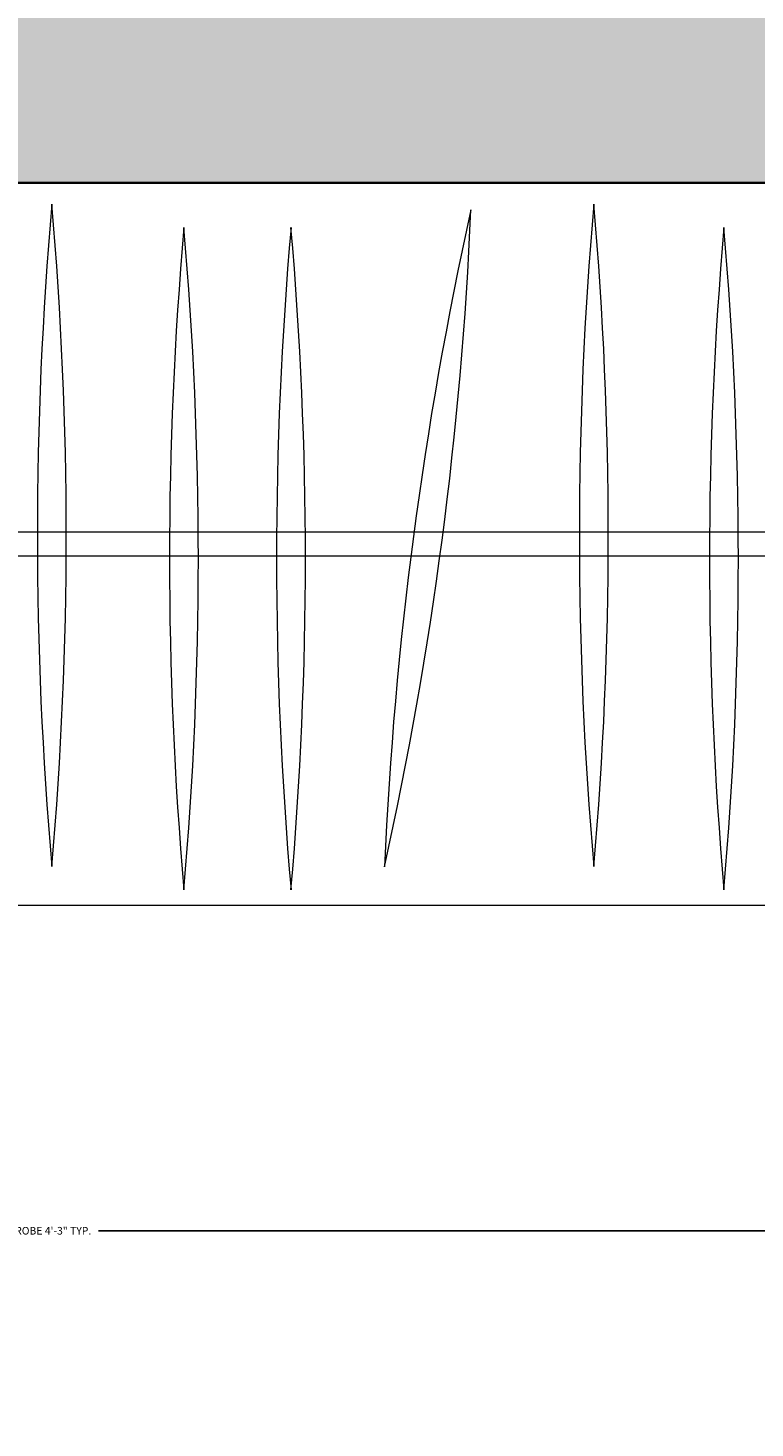
# Model space of a CAD drawing. Units: inches. Extents: x -9 to 505, y -680 to 48.
# Tile 10 of 17: x 62 to 79, y -198 to -165. Entities that reach past the tile are written whole.
import ezdxf

# ---------------------------------------------------------------- set-up
doc = ezdxf.new("R2010")
doc.units = ezdxf.units.IN
doc.header["$MEASUREMENT"] = 0
for name, color, linetype, lineweight in [('A-ANNO-DIMS', 2, 'Continuous', 18), ('A-FLOR-CASE', 8, 'Continuous', 18), ('A-WALL', 7, 'Continuous', 35), ('A-WALL-PATT', 251, 'Continuous', 13)]:
    doc.layers.add(name, color=color, linetype=linetype, lineweight=lineweight)
doc.styles.get("Standard").update_dxf_attribs({"font": 'arial.ttf'})
doc.dimstyles.get("Standard").update_dxf_attribs({"dimtxt": 0.18, "dimasz": 0.18, "dimexe": 0.18, "dimexo": 0.0625, "dimgap": 0.09, "dimtad": 0, "dimtih": 1, "dimtoh": 1, "dimdec": 0, "dimzin": 0, "dimdsep": 46, "dimlunit": 3, "dimtxsty": 'Standard', "dimcen": 0.09, "dimadec": 0, "dimazin": 0, "dimtfac": 1, "dimtdec": 0, "dimtofl": 0, "dimtmove": 0, "dimatfit": 3, "dimfxl": 1, "dimtolj": 1, "dimtzin": 0, "dimarcsym": 0})

# ---------------------------------------------------------------- blocks, each defined once
blk = doc.blocks.new('WARDROBE-HANGING')
for p, q in [((51.194, 17.065), (0, 17.065)), ((51.194, 8.817), (0, 8.817)), ((51.194, 8.248), (0, 8.248)), ((51.194, 0), (0, 0))]:
    blk.add_line(p, q)
for centre, start, end in [((115.358, 8.742), 175.00281, 184.99719), ((-63.542, 8.742), 355.00281, 4.99719), ((128.16, 8.742), 175.00281, 184.99719), ((-50.739, 8.742), 355.00281, 4.99719), ((123.474, -2.996), 167.50795, 177.50233), ((-53.897, 20.34), 347.50795, 357.50233), ((118.479, 8.192), 175.00281, 184.99719), ((-60.421, 8.192), 355.00281, 4.99719), ((121.008, 8.192), 175.00281, 184.99719), ((-57.892, 8.192), 355.00281, 4.99719), ((131.234, 8.192), 175.00281, 184.99719), ((-47.666, 8.192), 355.00281, 4.99719)]:
    blk.add_arc(centre, 89.791, start, end)
blk = doc.blocks.new('*D22')
at = {"layer": 'A-ANNO-DIMS', "color": 0, "lineweight": -2, "transparency": 16777216}
for p, q in [((36.264, -185.628), (36.264, -193.425)), ((87.458, -185.628), (87.458, -193.425)), ((36.444, -193.245), (60.443, -193.245)), ((87.278, -193.245), (63.279, -193.245))]:
    blk.add_line(p, q, dxfattribs=at)
at = {"layer": 'A-ANNO-DIMS', "color": 0, "transparency": 16777216}
for points in [[(36.444, -193.215), (36.444, -193.275), (36.264, -193.245)], [(87.278, -193.215), (87.278, -193.275), (87.458, -193.245)]]:
    blk.add_solid(points, dxfattribs=at)
at = {"layer": 'Defpoints', "color": 0, "transparency": 16777216}
for p in [(36.264, -185.566), (87.458, -185.566), (87.458, -193.245)]:
    blk.add_point(p, dxfattribs=at)
at = {"layer": 'A-ANNO-DIMS', "color": 0, "transparency": 16777216, "insert": (61.861, -193.245), "char_height": 0.18, "attachment_point": 5}
blk.add_mtext('\\A1;WARDROBE 4\'-3" TYP.', dxfattribs=at)

msp = doc.modelspace()

# ---------------------------------------------------------------- hatches: boundary and pattern name
at = {"layer": 'A-WALL-PATT'}
h = msp.add_hatch(color=256, dxfattribs=at)
h.dxf.hatch_style = 1
h.paths.add_polyline_path([(101.641, 11.499), (48.264, 11.499), (48.264, 2.499), (72.264, 2.499), (72.264, -21.248), (81.264, -21.248), (81.264, 2.499), (101.641, 2.499)])
h.paths.add_polyline_path([(36.264, 2.499), (27.264, 2.499), (27.264, -6.918), (36.264, -6.918)])
h.paths.add_polyline_path([(81.264, -57.248), (72.264, -57.248), (72.264, -75.501), (81.264, -75.501)])
h.paths.add_polyline_path([(162.764, 11.499), (137.641, 11.499), (137.641, 2.499), (162.764, 2.499)])
h.paths.add_polyline_path([(179.264, 2.499), (174.764, 2.499), (174.764, -75.501), (179.264, -75.501), (179.264, -54.501), (229.514, -54.501), (229.514, -45.501), (179.264, -45.501)])
h.paths.add_polyline_path([(382.256, -45.501), (332.264, -45.501), (332.264, 2.499), (327.764, 2.499), (327.764, -45.501), (277.514, -45.501), (277.514, -54.501), (327.764, -54.501), (327.764, -111.501), (332.264, -111.501), (332.264, -54.501), (382.256, -54.501)])
h.paths.add_polyline_path([(332.264, -128.001), (327.764, -128.001), (327.764, -207.001), (332.264, -207.001)])
h.paths.add_polyline_path([(124.764, -111.501), (36.264, -111.501), (36.264, -116.001), (120.264, -116.001), (120.264, -168.501), (179.264, -168.501), (179.264, -164.001), (124.764, -164.001)])
h.paths.add_polyline_path([(96.264, -164.001), (36.264, -164.001), (36.264, -152.001), (27.264, -152.001), (27.264, -208.879), (36.264, -208.879), (36.264, -168.501), (96.264, -168.501)])
h.paths.add_polyline_path([(36.264, -244.879), (27.264, -244.879), (27.264, -287.001), (36.264, -287.001)])
h.paths.add_polyline_path([(179.264, -204.501), (174.764, -204.501), (174.764, -287.001), (179.264, -287.001)])
h.paths.add_polyline_path([(257.264, -296.001), (248.264, -296.001), (248.264, -446.001), (269.264, -446.001), (269.264, -437.001), (257.264, -437.001)])
h.paths.add_polyline_path([(90.264, -296.001), (81.264, -296.001), (81.264, -348.67), (90.264, -348.67)])
h.paths.add_polyline_path([(90.264, -384.67), (81.264, -384.67), (81.264, -416.001), (90.264, -416.001)])
h.paths.add_polyline_path([(170.264, -452.001), (36.264, -452.001), (36.264, -456.501), (165.764, -456.501), (165.764, -504.501), (165.133, -504.501), (165.133, -509.001), (170.264, -509.001)])
h.paths.add_polyline_path([(141.764, -504.501), (36.264, -504.501), (36.264, -492.501), (27.264, -492.501), (27.264, -565.959), (36.264, -565.959), (36.264, -509.001), (141.764, -509.001)])
h.paths.add_polyline_path([(36.264, -601.959), (27.264, -601.959), (27.264, -658.501), (36.264, -658.501)])
h.paths.add_polyline_path([(170.264, -670.501), (170.264, -634.501), (222.764, -634.501), (222.764, -625.501), (165.764, -625.501), (165.764, -670.501), (36.264, -670.501), (36.264, -679.501), (170.264, -679.501)])
h.paths.add_polyline_path([(332.264, -616.501), (433.894, -616.501), (433.894, -612.001), (332.264, -612.001), (332.264, -610.563), (327.764, -610.563), (327.764, -625.501), (270.764, -625.501), (270.764, -634.501), (327.764, -634.501), (327.764, -658.501), (332.264, -658.501)])
h.paths.add_polyline_path([(459.764, -670.501), (336.764, -670.501), (336.764, -679.501), (459.764, -679.501)])
h.paths.add_polyline_path([(468.764, -545.737), (459.764, -545.737), (459.764, -612.001), (457.894, -612.001), (457.894, -616.501), (459.764, -616.501), (459.764, -658.501), (468.764, -658.501)])
h.paths.add_polyline_path([(332.264, -446.001), (327.764, -446.001), (327.764, -574.563), (332.264, -574.563)])
h.paths.add_polyline_path([(327.764, -437.001), (305.264, -437.001), (305.264, -446.001), (327.764, -446.001)])
h.paths.add_polyline_path([(459.764, -437.001), (348.764, -437.001), (348.764, -446.001), (459.764, -446.001)])
h.paths.add_polyline_path([(468.764, -458.001), (459.764, -458.001), (459.764, -509.737), (468.764, -509.737)])
h.paths.add_polyline_path([(468.764, -365.001), (459.764, -365.001), (459.764, -437.001), (468.764, -437.001)])
h.paths.add_polyline_path([(468.764, -299.601), (459.764, -299.601), (459.764, -344.001), (468.764, -344.001)])
h.paths.add_polyline_path([(468.764, -184.739), (459.764, -184.739), (459.764, -231.001), (401.264, -231.001), (401.264, -235.501), (459.764, -235.501), (459.764, -275.601), (468.764, -275.601)])
h.paths.add_polyline_path([(390.764, -356.001), (342.764, -356.001), (342.764, -365.001), (390.764, -365.001)])
h.paths.add_polyline_path([(459.764, -356.001), (405.764, -356.001), (405.764, -365.001), (459.764, -365.001)])
h.paths.add_polyline_path([(405.764, -296.001), (396.764, -296.001), (396.764, -356.001), (405.764, -356.001)])
h.paths.add_polyline_path([(336.764, -296.001), (327.764, -296.001), (327.764, -356.001), (336.764, -356.001)])
h.paths.add_polyline_path([(468.764, -9.501), (459.764, -9.501), (459.764, -45.501), (418.256, -45.501), (418.256, -54.501), (468.764, -54.501)])
h.paths.add_polyline_path([(468.764, -54.501), (459.764, -54.501), (459.764, -111.501), (468.764, -111.501)])
h.paths.add_polyline_path([(468.764, -128.001), (459.764, -128.001), (459.764, -148.739), (468.764, -148.739)])

# ---------------------------------------------------------------- linework, layer by layer
at = {"layer": 'A-WALL'}
msp.add_line((36.264, -168.501), (179.264, -168.501), dxfattribs=at)

# ---------------------------------------------------------------- block references
at = {"layer": 'A-FLOR-CASE'}
msp.add_blockref('WARDROBE-HANGING', (36.264, -185.566), dxfattribs=at)

# ---------------------------------------------------------------- dimensions: what is measured, and where the dimension line sits
at = {"layer": 'A-ANNO-DIMS'}
dim = msp.add_linear_dim(base=(87.458, -193.245), p1=(36.264, -185.566), p2=(87.458, -185.566), text='WARDROBE <> TYP.', dimstyle='Standard', override={"dimdec": 1, "dimlfac": 1, "dimrnd": 0, "dimzin": 1, "dimdsep": 46, "dimlunit": 4, "dimfrac": 2}, dxfattribs=at)
dim.commit()
dim.dimension.update_dxf_attribs({"geometry": '*D22', "text_midpoint": (61.861, -193.245)})

doc.saveas('drawing.dxf')
